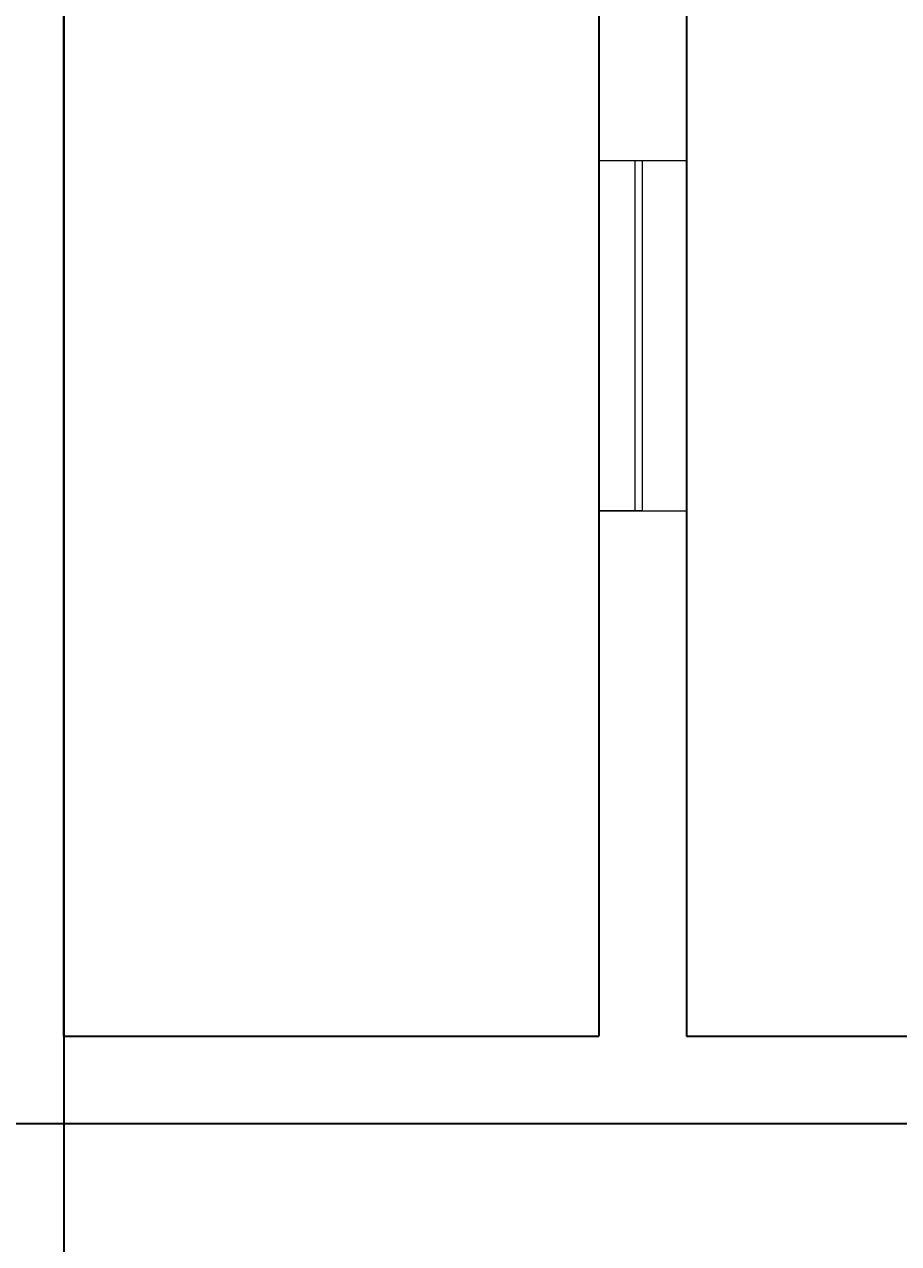
# Model space of a CAD drawing. Units: inches. Extents: x -61 to 1599, y -1316 to 257.
# Tile 185 of 204: x 998 to 1088, y -454 to -328. Entities that reach past the tile are written whole.
import ezdxf

# ---------------------------------------------------------------- set-up
doc = ezdxf.new("R2010")
doc.units = ezdxf.units.IN
doc.header["$MEASUREMENT"] = 0
for name, color, linetype, lineweight in [('A-ANNO-DIMS', 2, 'Continuous', 18), ('WALLS', 4, 'Continuous', 35), ('WINDOWS', 220, 'Continuous', 18)]:
    doc.layers.add(name, color=color, linetype=linetype, lineweight=lineweight)
doc.styles.get("Standard").update_dxf_attribs({"font": 'arial.ttf'})
doc.dimstyles.get("Standard").update_dxf_attribs({"dimtxt": 0.18, "dimasz": 0.18, "dimexe": 0.18, "dimexo": 0.0625, "dimgap": 0.09, "dimtad": 0, "dimtih": 1, "dimtoh": 1, "dimdec": 0, "dimzin": 0, "dimdsep": 46, "dimlunit": 3, "dimtxsty": 'Standard', "dimcen": 0.09, "dimadec": 0, "dimazin": 0, "dimtfac": 1, "dimtdec": 0, "dimtofl": 0, "dimtmove": 0, "dimatfit": 3, "dimfxl": 1, "dimtolj": 1, "dimtzin": 0, "dimarcsym": 0})

# ---------------------------------------------------------------- blocks, each defined once
blk = doc.blocks.new('WIN-36IN')
for p, q in [((0, 4.5), (0, 9)), ((0, 9), (0, 0)), ((36, 9), (36, 0)), ((0, 5.26), (36, 5.26)), ((0, 4.5), (36, 4.5)), ((0, 4.5), (36, 4.5))]:
    blk.add_line(p, q)
blk = doc.blocks.new('*D698')
at = {"layer": 'A-ANNO-DIMS', "color": 0, "lineweight": -2, "transparency": 16777216}
for p, q in [((644.77, -167.17), (1598.48, -167.17)), ((1598.3, -167.35), (1598.3, -363.99)), ((1598.3, -560.99), (1598.3, -364.35)), ((644.77, -561.17), (1598.48, -561.17))]:
    blk.add_line(p, q, dxfattribs=at)
at = {"layer": 'A-ANNO-DIMS', "color": 0, "transparency": 16777216}
for points in [[(1598.27, -167.35), (1598.33, -167.35), (1598.3, -167.17)], [(1598.27, -560.99), (1598.33, -560.99), (1598.3, -561.17)]]:
    blk.add_solid(points, dxfattribs=at)
at = {"layer": 'DEFPOINTS', "color": 0, "transparency": 16777216}
for p in [(644.7, -167.17), (1598.3, -167.17), (644.7, -561.17)]:
    blk.add_point(p, dxfattribs=at)
at = {"layer": 'A-ANNO-DIMS', "color": 0, "transparency": 16777216, "insert": (1598.3, -364.17), "char_height": 0.18, "attachment_point": 5}
blk.add_mtext('\\A1;394', dxfattribs=at)

msp = doc.modelspace()

# ---------------------------------------------------------------- linework, layer by layer
at = {"layer": 'WALLS'}
for p, q in [((1001.7028, -175.3229), (1001.7028, -432.3229)), ((1056.7028, -175.3229), (1056.7028, -432.3229)), ((1001.7028, -432.3229), (1001.7028, -289.3229)), ((1065.7028, -288.3229), (1065.7028, -432.3229)), ((1001.7028, -432.3229), (1001.7028, -741.169)), ((1001.7028, -432.3229), (1056.7028, -432.3229)), ((1065.7028, -432.3229), (1215.7028, -432.3229)), ((992.7028, -441.3229), (1215.7028, -441.3229))]:
    msp.add_line(p, q, dxfattribs=at)

# ---------------------------------------------------------------- block references
at = {"layer": 'WINDOWS', "rotation": 89.99999999999925}
msp.add_blockref('WIN-36IN', (1065.7029, -378.3189), dxfattribs=at)

# ---------------------------------------------------------------- dimensions: what is measured, and where the dimension line sits
at = {"layer": 'A-ANNO-DIMS'}
dim = msp.add_linear_dim(base=(1598.3028, -167.169), p1=(644.7028, -561.169), p2=(644.7028, -167.169), angle=90, dimstyle='Standard', override={"dimdec": 0, "dimlfac": 1, "dimrnd": 0, "dimzin": 0, "dimdsep": 46, "dimlunit": 2}, dxfattribs=at)
dim.commit()
dim.dimension.update_dxf_attribs({"geometry": '*D698', "text_midpoint": (1598.3028, -364.169)})

doc.saveas('drawing.dxf')
